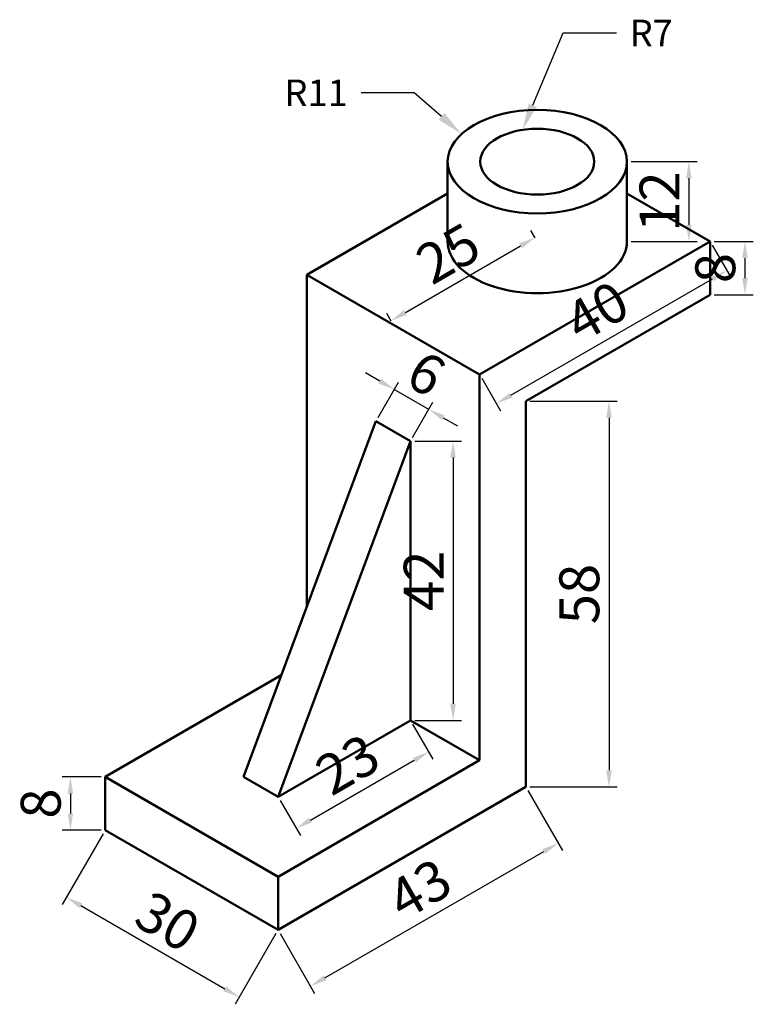
# Model space of a CAD drawing. Units: millimetres. Extents: x 3714 to 3825, y 1185 to 1333.
import ezdxf
from ezdxf import colors
from ezdxf.entities.mleader import LeaderData, LeaderLine
from ezdxf.math import Vec2, Vec3

# ---------------------------------------------------------------- set-up
doc = ezdxf.new("R2010")
doc.units = ezdxf.units.MM
for name, color, linetype, lineweight in [('M-DIMS', 2, 'Continuous', 25), ('M-OUTL', 7, 'Continuous', 50), ('M-TEXT', 3, 'Continuous', 25)]:
    doc.layers.add(name, color=color, linetype=linetype, lineweight=lineweight)
doc.styles.get("Standard").update_dxf_attribs({"font": 'arial.ttf'})
doc.dimstyles.new('ISO-25', dxfattribs={"dimtxt": 6, "dimasz": 2.5, "dimexe": 1.25, "dimexo": 0.625, "dimtad": 1, "dimtxsty": 'Standard', "dimcen": 2.5, "dimadec": 0, "dimazin": 0, "dimtfac": 1, "dimtmove": 0, "dimatfit": 3, "dimfxl": 1, "dimarcsym": 0})

# ---------------------------------------------------------------- blocks, each defined once
blk = doc.blocks.new('*D1')
at = {"layer": 'Defpoints', "color": 0, "transparency": 16777216}
for p in [(3790.43, 1217.21), (3795.31, 1208.75), (3753.19, 1195.71)]:
    blk.add_point(p, dxfattribs=at)
at = {"layer": 'M-DIMS', "color": 0, "lineweight": -2, "transparency": 16777216}
for p, q in [((3790.74, 1216.67), (3795.94, 1207.67)), ((3760.24, 1188.5), (3793.15, 1207.5)), ((3753.51, 1195.17), (3758.7, 1186.17))]:
    blk.add_line(p, q, dxfattribs=at)
at = {"layer": 'M-DIMS', "color": 0, "transparency": 16777216}
for points in [[(3792.94, 1207.86), (3793.36, 1207.14), (3795.31, 1208.75)], [(3760.03, 1188.86), (3760.45, 1188.14), (3758.08, 1187.25)]]:
    blk.add_solid(points, dxfattribs=at)
at = {"layer": 'M-DIMS', "color": 0, "transparency": 16777216, "insert": (3774.85, 1201.2), "char_height": 6, "attachment_point": 5, "rotation": 30}
blk.add_mtext('43', dxfattribs=at)
blk = doc.blocks.new('*D2')
at = {"layer": 'Defpoints', "color": 0, "transparency": 16777216}
for p in [(3727.21, 1210.71), (3753.19, 1195.71), (3747.36, 1185.61)]:
    blk.add_point(p, dxfattribs=at)
at = {"layer": 'M-DIMS', "color": 0, "lineweight": -2, "transparency": 16777216}
for p, q in [((3726.9, 1210.17), (3720.76, 1199.53)), ((3723.55, 1199.36), (3745.2, 1186.86)), ((3752.88, 1195.17), (3746.74, 1184.53))]:
    blk.add_line(p, q, dxfattribs=at)
at = {"layer": 'M-DIMS', "color": 0, "transparency": 16777216}
for points in [[(3723.76, 1199.72), (3723.34, 1199), (3721.38, 1200.61)], [(3745.41, 1187.22), (3744.99, 1186.5), (3747.36, 1185.61)]]:
    blk.add_solid(points, dxfattribs=at)
at = {"layer": 'M-DIMS', "color": 0, "transparency": 16777216, "insert": (3736.22, 1196.31), "char_height": 6, "attachment_point": 5, "rotation": 330}
blk.add_mtext('30', dxfattribs=at)
blk = doc.blocks.new('*D3')
at = {"layer": 'Defpoints', "color": 0, "transparency": 16777216}
for p in [(3727.21, 1218.71), (3721.98, 1210.71), (3727.21, 1210.71)]:
    blk.add_point(p, dxfattribs=at)
at = {"layer": 'M-DIMS', "color": 0, "lineweight": -2, "transparency": 16777216}
for p, q in [((3726.59, 1218.71), (3720.73, 1218.71)), ((3721.98, 1216.21), (3721.98, 1213.21)), ((3726.59, 1210.71), (3720.73, 1210.71))]:
    blk.add_line(p, q, dxfattribs=at)
at = {"layer": 'M-DIMS', "color": 0, "transparency": 16777216}
for points in [[(3721.57, 1216.21), (3722.4, 1216.21), (3721.98, 1218.71)], [(3721.57, 1213.21), (3722.4, 1213.21), (3721.98, 1210.71)]]:
    blk.add_solid(points, dxfattribs=at)
at = {"layer": 'M-DIMS', "color": 0, "transparency": 16777216, "insert": (3718.29, 1214.71), "char_height": 6, "attachment_point": 5, "rotation": 90}
blk.add_mtext('8', dxfattribs=at)
blk = doc.blocks.new('*D4')
at = {"layer": 'Defpoints', "color": 0, "transparency": 16777216}
for p in [(3790.43, 1275.21), (3790.43, 1217.21), (3802.95, 1217.21)]:
    blk.add_point(p, dxfattribs=at)
at = {"layer": 'M-DIMS', "color": 0, "lineweight": -2, "transparency": 16777216}
for p, q in [((3791.06, 1275.21), (3804.2, 1275.21)), ((3802.95, 1272.71), (3802.95, 1219.71)), ((3791.06, 1217.21), (3804.2, 1217.21))]:
    blk.add_line(p, q, dxfattribs=at)
at = {"layer": 'M-DIMS', "color": 0, "transparency": 16777216}
for points in [[(3802.53, 1272.71), (3803.37, 1272.71), (3802.95, 1275.21)], [(3802.53, 1219.71), (3803.37, 1219.71), (3802.95, 1217.21)]]:
    blk.add_solid(points, dxfattribs=at)
at = {"layer": 'M-DIMS', "color": 0, "transparency": 16777216, "insert": (3799.26, 1246.21), "char_height": 6, "attachment_point": 5, "rotation": 90}
blk.add_mtext('58', dxfattribs=at)
blk = doc.blocks.new('*D5')
at = {"layer": 'Defpoints', "color": 0, "transparency": 16777216}
for p in [(3818.14, 1299.21), (3820.67, 1294.84), (3783.5, 1279.21)]:
    blk.add_point(p, dxfattribs=at)
at = {"layer": 'M-DIMS', "color": 0, "lineweight": -2, "transparency": 16777216}
for p, q in [((3818.46, 1298.67), (3821.29, 1293.76)), ((3788.19, 1276.09), (3818.5, 1293.59)), ((3783.82, 1278.67), (3786.65, 1273.76))]:
    blk.add_line(p, q, dxfattribs=at)
at = {"layer": 'M-DIMS', "color": 0, "transparency": 16777216}
for points in [[(3818.29, 1293.95), (3818.71, 1293.23), (3820.67, 1294.84)], [(3787.98, 1276.45), (3788.4, 1275.73), (3786.03, 1274.84)]]:
    blk.add_solid(points, dxfattribs=at)
at = {"layer": 'M-DIMS', "color": 0, "transparency": 16777216, "insert": (3801.5, 1288.03), "char_height": 6, "attachment_point": 5, "rotation": 30}
blk.add_mtext('40', dxfattribs=at)
blk = doc.blocks.new('*D6')
at = {"layer": 'Defpoints', "color": 0, "transparency": 16777216}
for p in [(3818.14, 1299.21), (3818.14, 1291.21), (3823.39, 1291.21)]:
    blk.add_point(p, dxfattribs=at)
at = {"layer": 'M-DIMS', "color": 0, "lineweight": -2, "transparency": 16777216}
for p, q in [((3818.77, 1299.21), (3824.64, 1299.21)), ((3823.39, 1296.71), (3823.39, 1293.71)), ((3818.77, 1291.21), (3824.64, 1291.21))]:
    blk.add_line(p, q, dxfattribs=at)
at = {"layer": 'M-DIMS', "color": 0, "transparency": 16777216}
for points in [[(3822.98, 1296.71), (3823.81, 1296.71), (3823.39, 1299.21)], [(3822.98, 1293.71), (3823.81, 1293.71), (3823.39, 1291.21)]]:
    blk.add_solid(points, dxfattribs=at)
at = {"layer": 'M-DIMS', "color": 0, "transparency": 16777216, "insert": (3819.7, 1295.21), "char_height": 6, "attachment_point": 5, "rotation": 90}
blk.add_mtext('8', dxfattribs=at)
blk = doc.blocks.new('*D7')
at = {"layer": 'Defpoints', "color": 0, "transparency": 16777216}
for p in [(3770.66, 1276.97), (3767.92, 1272.21), (3773.11, 1269.21)]:
    blk.add_point(p, dxfattribs=at)
at = {"layer": 'M-DIMS', "color": 0, "lineweight": -2, "transparency": 16777216}
for p, q in [((3768.5, 1278.22), (3766.33, 1279.47)), ((3768.23, 1272.75), (3771.29, 1278.05)), ((3775.86, 1273.97), (3770.66, 1276.97)), ((3773.42, 1269.75), (3776.48, 1275.05)), ((3778.02, 1272.72), (3780.19, 1271.47))]:
    blk.add_line(p, q, dxfattribs=at)
at = {"layer": 'M-DIMS', "color": 0, "transparency": 16777216}
for points in [[(3768.71, 1278.58), (3768.29, 1277.86), (3770.66, 1276.97)], [(3778.23, 1273.08), (3777.82, 1272.36), (3775.86, 1273.97)]]:
    blk.add_solid(points, dxfattribs=at)
at = {"layer": 'M-DIMS', "color": 0, "transparency": 16777216, "insert": (3775.1, 1278.66), "char_height": 6, "attachment_point": 5, "rotation": 330}
blk.add_mtext('6', dxfattribs=at)
blk = doc.blocks.new('*D8')
at = {"layer": 'Defpoints', "color": 0, "transparency": 16777216}
for p in [(3773.11, 1269.21), (3773.11, 1227.21), (3779.51, 1227.21)]:
    blk.add_point(p, dxfattribs=at)
at = {"layer": 'M-DIMS', "color": 0, "lineweight": -2, "transparency": 16777216}
for p, q in [((3773.74, 1269.21), (3780.76, 1269.21)), ((3779.51, 1266.71), (3779.51, 1229.71)), ((3773.74, 1227.21), (3780.76, 1227.21))]:
    blk.add_line(p, q, dxfattribs=at)
at = {"layer": 'M-DIMS', "color": 0, "transparency": 16777216}
for points in [[(3779.09, 1266.71), (3779.92, 1266.71), (3779.51, 1269.21)], [(3779.09, 1229.71), (3779.92, 1229.71), (3779.51, 1227.21)]]:
    blk.add_solid(points, dxfattribs=at)
at = {"layer": 'M-DIMS', "color": 0, "transparency": 16777216, "insert": (3775.87, 1248.21), "char_height": 6, "attachment_point": 5, "rotation": 90}
blk.add_mtext('42', dxfattribs=at)
blk = doc.blocks.new('*D9')
at = {"layer": 'Defpoints', "color": 0, "transparency": 16777216}
for p in [(3773.11, 1227.21), (3775.84, 1222.48), (3753.19, 1215.71)]:
    blk.add_point(p, dxfattribs=at)
at = {"layer": 'M-DIMS', "color": 0, "lineweight": -2, "transparency": 16777216}
for p, q in [((3773.42, 1226.67), (3776.47, 1221.39)), ((3758.09, 1212.23), (3773.68, 1221.23)), ((3753.51, 1215.17), (3756.55, 1209.89))]:
    blk.add_line(p, q, dxfattribs=at)
at = {"layer": 'M-DIMS', "color": 0, "transparency": 16777216}
for points in [[(3773.47, 1221.59), (3773.89, 1220.87), (3775.84, 1222.48)], [(3757.88, 1212.59), (3758.3, 1211.87), (3755.92, 1210.98)]]:
    blk.add_solid(points, dxfattribs=at)
at = {"layer": 'M-DIMS', "color": 0, "transparency": 16777216, "insert": (3764.04, 1219.92), "char_height": 6, "attachment_point": 5, "rotation": 30}
blk.add_mtext('23', dxfattribs=at)
blk = doc.blocks.new('*D10')
at = {"layer": 'Defpoints', "color": 0, "transparency": 16777216}
for p in [(3791.82, 1299.8), (3792.16, 1299.21), (3770.51, 1286.71)]:
    blk.add_point(p, dxfattribs=at)
at = {"layer": 'M-DIMS', "color": 0, "lineweight": -2, "transparency": 16777216}
for p, q in [((3791.85, 1299.75), (3791.2, 1300.88)), ((3772.34, 1288.55), (3789.66, 1298.55)), ((3770.2, 1287.25), (3769.55, 1288.38))]:
    blk.add_line(p, q, dxfattribs=at)
at = {"layer": 'M-DIMS', "color": 0, "transparency": 16777216}
for points in [[(3789.45, 1298.91), (3789.87, 1298.19), (3791.82, 1299.8)], [(3772.13, 1288.91), (3772.55, 1288.19), (3770.17, 1287.3)]]:
    blk.add_solid(points, dxfattribs=at)
at = {"layer": 'M-DIMS', "color": 0, "transparency": 16777216, "insert": (3779.16, 1296.74), "char_height": 6, "attachment_point": 5, "rotation": 30}
blk.add_mtext('25', dxfattribs=at)
blk = doc.blocks.new('*D11')
at = {"layer": 'Defpoints', "color": 0, "transparency": 16777216}
for p in [(3805.64, 1311.21), (3805.64, 1299.21), (3814.95, 1299.21)]:
    blk.add_point(p, dxfattribs=at)
at = {"layer": 'M-DIMS', "color": 0, "lineweight": -2, "transparency": 16777216}
for p, q in [((3806.26, 1311.21), (3816.2, 1311.21)), ((3814.95, 1308.71), (3814.95, 1301.71)), ((3806.26, 1299.21), (3816.2, 1299.21))]:
    blk.add_line(p, q, dxfattribs=at)
at = {"layer": 'M-DIMS', "color": 0, "transparency": 16777216}
for points in [[(3814.54, 1308.71), (3815.37, 1308.71), (3814.95, 1311.21)], [(3814.54, 1301.71), (3815.37, 1301.71), (3814.95, 1299.21)]]:
    blk.add_solid(points, dxfattribs=at)
at = {"layer": 'M-DIMS', "color": 0, "transparency": 16777216, "insert": (3811.32, 1305.21), "char_height": 6, "attachment_point": 5, "rotation": 90}
blk.add_mtext('12', dxfattribs=at)

msp = doc.modelspace()

# ---------------------------------------------------------------- linework, layer by layer
at = {"layer": 'M-OUTL'}
for p, q in [((3778.692, 1299.209), (3778.692, 1311.209)), ((3805.636, 1299.209), (3805.636, 1311.209)), ((3757.523, 1294.209), (3778.692, 1306.431)), ((3805.636, 1306.431), (3818.145, 1299.209)), ((3818.145, 1299.209), (3783.504, 1279.209)), ((3818.145, 1299.209), (3818.145, 1291.209)), ((3783.504, 1279.209), (3757.523, 1294.209)), ((3757.523, 1294.209), (3757.523, 1244.296)), ((3818.145, 1291.209), (3790.432, 1275.209)), ((3783.504, 1221.209), (3783.504, 1279.209)), ((3790.432, 1275.209), (3790.432, 1217.209)), ((3747.997, 1218.709), (3767.915, 1272.209)), ((3767.915, 1272.209), (3773.112, 1269.209)), ((3770.513, 1270.709), (3773.112, 1269.209)), ((3773.112, 1269.209), (3753.193, 1215.709)), ((3773.112, 1269.209), (3773.112, 1227.209)), ((3753.688, 1233.995), (3727.212, 1218.709)), ((3773.112, 1227.209), (3753.193, 1215.709)), ((3773.112, 1227.209), (3783.504, 1221.209)), ((3753.193, 1203.709), (3783.504, 1221.209)), ((3727.212, 1218.709), (3753.193, 1203.709)), ((3727.212, 1210.709), (3727.212, 1218.709)), ((3753.193, 1215.709), (3747.997, 1218.709)), ((3753.193, 1215.709), (3747.997, 1218.709)), ((3790.432, 1217.209), (3753.193, 1195.709)), ((3753.193, 1195.709), (3727.212, 1210.709)), ((3753.193, 1195.709), (3753.193, 1203.709))]:
    msp.add_line(p, q, dxfattribs=at)
for major_axis in [(-13.472, 0), (-8.573, 0)]:
    msp.add_ellipse((3792.164, 1311.209), major_axis=major_axis, ratio=0.5773503, dxfattribs=at)
msp.add_ellipse((3792.164, 1299.209), major_axis=(-13.472, 0), ratio=0.5773503, start_param=0, end_param=3.1415927, dxfattribs=at)

# ---------------------------------------------------------------- dimensions: what is measured, and where the dimension line sits
at = {"layer": 'M-DIMS'}
for p1, p2, distance, picture, middle in [((3805.636, 1311.209), (3805.636, 1299.209), 9.317, '*D11', (3811.316, 1305.209)), ((3770.513, 1286.709), (3792.164, 1299.209), 0.679, '*D10', (3779.155, 1296.742)), ((3783.504, 1279.209), (3818.145, 1299.209), -5.046, '*D5', (3801.503, 1288.033)), ((3818.145, 1299.209), (3818.145, 1291.209), 5.248, '*D6', (3819.704, 1295.209)), ((3773.112, 1269.209), (3767.915, 1272.209), -5.494, '*D7', (3775.105, 1278.662)), ((3790.432, 1275.209), (3790.432, 1217.209), 12.518, '*D4', (3799.262, 1246.209)), ((3773.112, 1269.209), (3773.112, 1227.209), 6.396, '*D8', (3775.871, 1248.209)), ((3753.193, 1215.709), (3773.112, 1227.209), -5.464, '*D9', (3764.039, 1219.924)), ((3753.193, 1195.709), (3790.432, 1217.209), -9.766, '*D1', (3774.85, 1201.198)), ((3727.212, 1210.709), (3753.193, 1195.709), -11.659, '*D2', (3736.218, 1196.309))]:
    dim = msp.add_aligned_dim(p1=p1, p2=p2, distance=distance, dimstyle='ISO-25', override={"dimclrd": 0, "dimclre": 0, "dimclrt": 0}, dxfattribs=at)
    dim.commit()
    dim.dimension.update_dxf_attribs({"geometry": picture, "text_midpoint": middle})
dim = msp.add_linear_dim(base=(3721.982, 1210.709), p1=(3727.212, 1218.709), p2=(3727.212, 1210.709), angle=90, dimstyle='ISO-25', override={"dimclrd": 0, "dimclre": 0, "dimclrt": 0}, dxfattribs=at)
dim.commit()
dim.dimension.update_dxf_attribs({"geometry": '*D3', "text_midpoint": (3718.293, 1214.709)})

# ---------------------------------------------------------------- leaders
at = {"layer": 'M-TEXT'}
ml = msp.add_multileader_mtext('Standard', dxfattribs=at)
ml.set_content('R7', color=256)
ml.set_leader_properties()
ml.build(insert=Vec2(0, 0))
ctx = ml.context
ctx.base_point, ctx.plane_origin = Vec3(3804.054, 1330.552), Vec3(3789.94, 1315.99)
notes = []
notes.append((ctx, [(0, (1, 1, 0), (3796.054, 1330.552), (1, 0), 8, [(0, [(3789.94, 1315.99)], 0, [])])]))
ctx.mtext.insert, ctx.mtext.flow_direction = Vec3(3806.054, 1332.552), 5
ml = msp.add_multileader_mtext('Standard', dxfattribs=at)
ml.set_content('R11', color=256)
ml.set_leader_properties()
ml.build(insert=Vec2(0, 0))
ctx = ml.context
ctx.base_point, ctx.plane_origin = Vec3(3752.897, 1321.557), Vec3(3780.788, 1315.376)
ctx.text_align_type = 2
notes.append((ctx, [(0, (1, 1, 0), (3773.682, 1321.557), (-1, 0), 8, [(0, [(3780.788, 1315.376)], 0, [])])]))
ctx.mtext.insert, ctx.mtext.alignment, ctx.mtext.flow_direction = Vec3(3763.682, 1323.557), 3, 5
for ctx, leaders in notes:
    for number, flags, end, landing, length, lines in leaders:
        leader = LeaderData()
        leader.index, (leader.has_last_leader_line, leader.has_dogleg_vector, leader.attachment_direction) = number, flags
        leader.last_leader_point, leader.dogleg_vector, leader.dogleg_length = Vec3(end), Vec3(landing), length
        for number, points, colour, breaks in lines:
            line = LeaderLine()
            line.index, line.vertices, line.color, line.breaks = number, Vec3.list(points), colors.encode_raw_color(colour), breaks
            leader.lines.append(line)
        ctx.leaders.append(leader)

doc.saveas('drawing.dxf')
